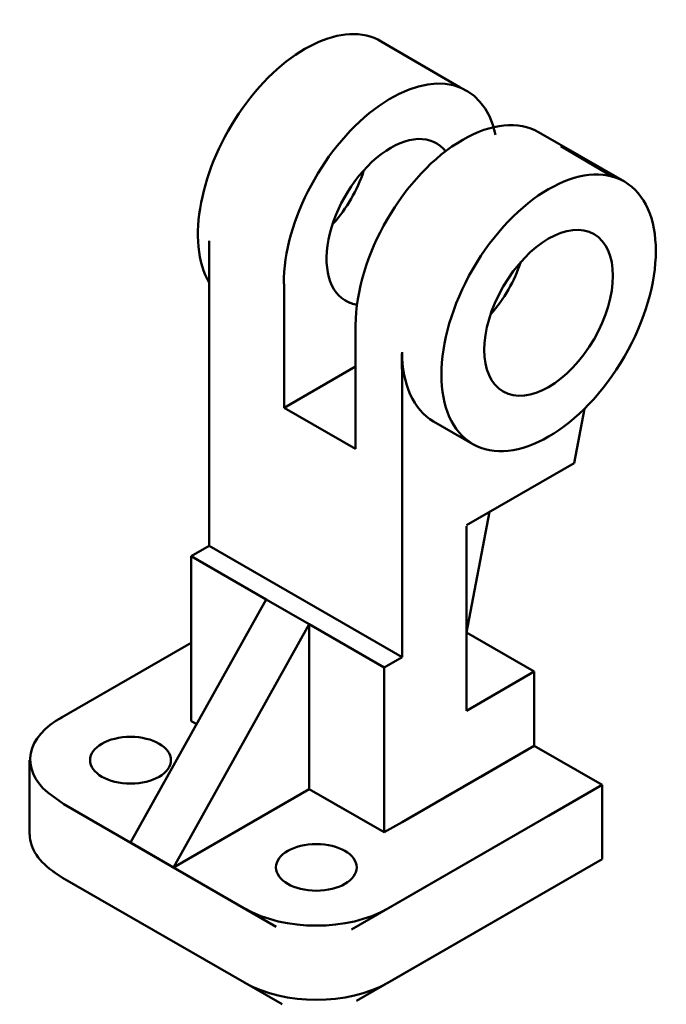
# Model space of a CAD drawing. Units: millimetres. Extents: x 53373983 to 53374139, y 67816294 to 67816533.
import ezdxf

# ---------------------------------------------------------------- set-up
doc = ezdxf.new("R2010")
doc.units = ezdxf.units.MM
doc.layers.add('M-OUTL', color=7, linetype='Continuous', lineweight=50)

msp = doc.modelspace()

# ---------------------------------------------------------------- linework, layer by layer
at = {"layer": 'M-OUTL'}
for p, q in [((53374089.29, 67816516.23), (53374070.15, 67816527.43)), ((53374129.09, 67816493.4), (53374108.31, 67816505.4)), ((53374126.31, 67816494.58), (53374113.65, 67816501.98)), ((53374028.45, 67816449.08), (53374028.45, 67816479.08)), ((53374046.64, 67816468.58), (53374046.64, 67816438.58)), ((53374063.96, 67816458.58), (53374063.96, 67816428.58)), ((53374075.22, 67816419.66), (53374075.22, 67816452.08)), ((53374075.22, 67816452.08), (53374075.22, 67816412.08)), ((53374028.45, 67816405.08), (53374028.45, 67816449.08)), ((53374046.64, 67816438.58), (53374063.96, 67816448.58)), ((53374063.96, 67816428.58), (53374046.64, 67816438.58)), ((53374116.89, 67816425.14), (53374119.4, 67816438.31)), ((53374092.35, 67816429.76), (53374082.83, 67816435.26)), ((53374090.81, 67816410.08), (53374116.89, 67816425.14)), ((53374075.22, 67816378.08), (53374075.22, 67816419.66)), ((53374090.81, 67816384.08), (53374096.37, 67816413.29)), ((53374075.22, 67816412.08), (53374075.22, 67816378.08)), ((53374090.81, 67816404.08), (53374090.81, 67816409.83)), ((53374024.12, 67816402.58), (53374028.45, 67816405.08)), ((53374075.22, 67816378.08), (53374028.45, 67816405.08)), ((53374090.81, 67816365.08), (53374090.81, 67816404.08)), ((53374042.31, 67816392.08), (53374024.12, 67816402.58)), ((53374024.12, 67816402.58), (53374024.12, 67816362.58)), ((53374009.4, 67816333.08), (53374042.31, 67816392.08)), ((53374052.7, 67816386.08), (53374042.31, 67816392.08)), ((53374019.79, 67816327.08), (53374052.7, 67816386.08)), ((53374052.7, 67816346.08), (53374052.7, 67816386.08)), ((53374052.7, 67816386.08), (53374070.89, 67816375.58)), ((53374107.26, 67816374.58), (53374090.81, 67816384.08)), ((53373991.69, 67816362.85), (53374024.12, 67816381.58)), ((53374070.89, 67816375.58), (53374075.22, 67816378.08)), ((53374070.89, 67816335.58), (53374070.89, 67816375.58)), ((53374070.89, 67816335.58), (53374070.89, 67816375.58)), ((53374107.26, 67816374.58), (53374090.81, 67816365.08)), ((53374105.53, 67816373.58), (53374107.26, 67816374.58)), ((53374105.53, 67816373.58), (53374107.26, 67816374.58)), ((53374107.26, 67816356.58), (53374107.26, 67816374.58)), ((53374024.12, 67816362.58), (53374025.43, 67816361.82)), ((53374075.22, 67816338.08), (53374107.26, 67816356.58)), ((53374107.26, 67816356.58), (53374075.22, 67816338.08)), ((53374075.22, 67816338.08), (53374107.26, 67816356.58)), ((53374107.26, 67816356.58), (53374079.55, 67816340.58)), ((53374107.26, 67816356.58), (53374089.94, 67816346.58)), ((53374094.27, 67816349.08), (53374105.53, 67816355.58)), ((53374105.53, 67816355.58), (53374107.26, 67816356.58)), ((53374107.26, 67816356.58), (53374123.71, 67816347.08)), ((53373984.9, 67816335.08), (53373984.9, 67816353.08)), ((53374094.27, 67816349.08), (53374075.22, 67816338.08)), ((53374094.27, 67816349.08), (53374085.61, 67816344.08)), ((53374052.7, 67816346.08), (53374019.79, 67816327.08)), ((53374070.89, 67816335.58), (53374052.7, 67816346.08)), ((53374052.7, 67816346.08), (53374061.79, 67816340.83)), ((53374123.71, 67816347.08), (53374062.97, 67816312.01)), ((53374123.71, 67816347.08), (53374062.97, 67816312.01)), ((53374123.71, 67816347.08), (53374071.75, 67816317.08)), ((53374110.72, 67816339.58), (53374123.71, 67816347.08)), ((53374123.71, 67816347.08), (53374123.71, 67816329.08)), ((53373989.36, 67816345.23), (53373993.27, 67816342.39)), ((53374044.72, 67816312.68), (53373993.27, 67816342.39)), ((53374075.22, 67816338.08), (53374078.68, 67816340.08)), ((53374075.22, 67816338.08), (53374070.89, 67816335.58)), ((53373984.92, 67816335.08), (53373984.96, 67816335.08)), ((53374019.79, 67816327.08), (53374009.4, 67816333.08)), ((53374019.79, 67816327.08), (53374009.4, 67816333.08)), ((53374123.71, 67816329.08), (53374064.14, 67816294.68)), ((53374123.71, 67816329.08), (53374064.14, 67816294.68)), ((53374123.71, 67816329.08), (53374064.14, 67816294.68)), ((53374123.71, 67816329.08), (53374071.75, 67816299.08)), ((53374123.69, 67816329.07), (53374123.71, 67816329.08)), ((53373990.68, 67816326.09), (53373992.95, 67816324.58)), ((53374046.14, 67816293.87), (53373992.95, 67816324.58))]:
    msp.add_line(p, q, dxfattribs=at)
msp.add_arc((53374099.82, 67816449.82), 24.71, 174.756, 185.244, dxfattribs=at)
for centre, major_axis, start_param, end_param in [((53374051.72, 67816495.64), (-18.37, -31.82), 3.138299, 5.958889), ((53374072.5, 67816483.64), (-18.37, -31.82), 2.575061, 5.497787), ((53374089.94, 67816473.58), (18.37, 31.82), 0, 0.785398), ((53374072.5, 67816483.64), (-11.02, -19.09), 2.906527, 6.421173), ((53374089.94, 67816473.58), (18.37, 31.82), 0.785398, 2.356194), ((53374051.83, 67816495.58), (11.02, 19.09), 4.372552, 5.052226), ((53374089.94, 67816473.58), (11.02, 19.09), 4.372552, 5.052226), ((53374072.62, 67816483.58), (11.02, 19.09), 3.141593, 3.363396), ((53374101.2, 67816467.08), (18.37, 31.82), 2.356194, 3.141593), ((53374009.59, 67816353.2), (-24.49, 0), 5.463741, 6.882182), ((53374009.46, 67816335.17), (-24.49, 0), 6.289909, 7.010692), ((53374054.43, 67816327.08), (24.49, 0), 3.926991, 5.497787), ((53374054.43, 67816309.08), (24.49, 0), 3.926991, 5.497787)]:
    msp.add_ellipse(centre, major_axis=major_axis, ratio=0.57735, start_param=start_param, end_param=end_param, dxfattribs=at)
for centre, major_axis in [((53374110.72, 67816461.58), (-18.37, -31.82)), ((53374110.72, 67816461.58), (-18.37, -31.82)), ((53374110.72, 67816461.58), (-18.37, -31.82)), ((53374110.72, 67816461.58), (-11.02, -19.09)), ((53374009.4, 67816353.08), (-9.8, 0)), ((53374054.43, 67816327.08), (-9.8, 0))]:
    msp.add_ellipse(centre, major_axis=major_axis, ratio=0.57735, dxfattribs=at)

doc.saveas('drawing.dxf')
